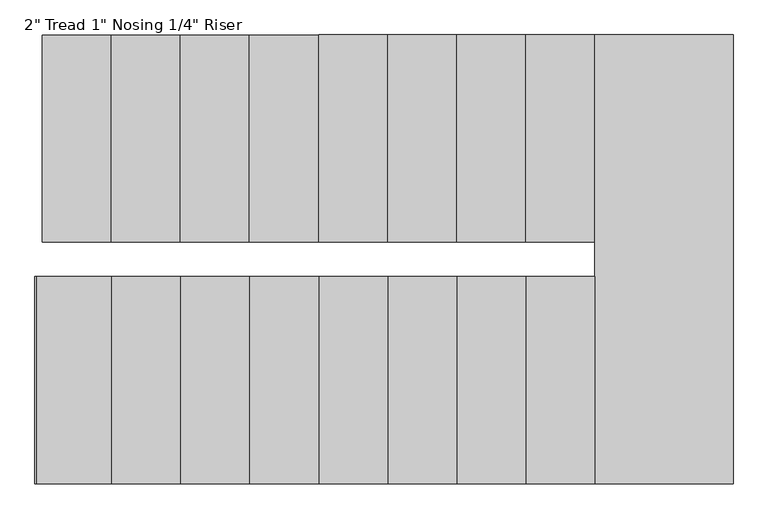
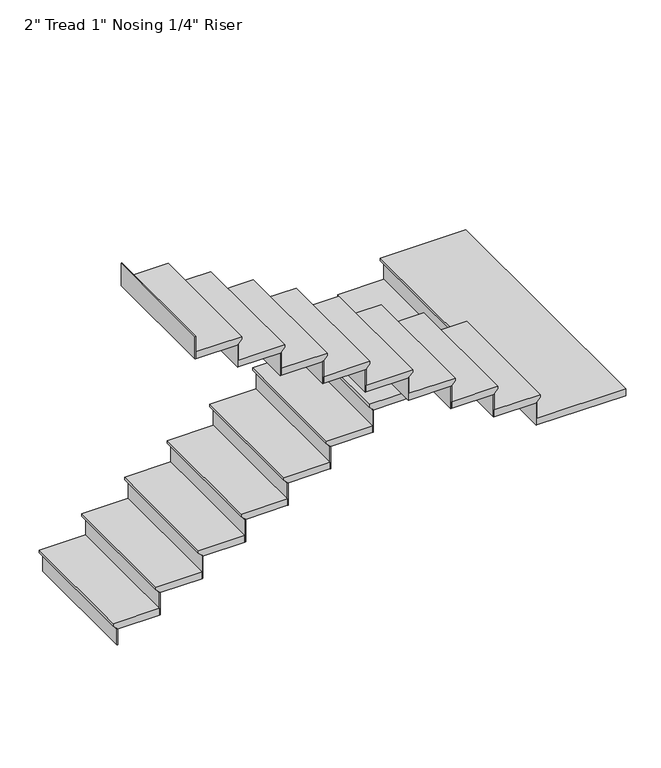
"""IFC4 building model written with IfcOpenShell, lengths in millimetres: stair flight geometry."""

from ifc_helpers import new_model, si_unit, origin, place, context, project, spatial, faceted_brep, source, transform, mapped, element, save


def stair_flight_0ccda8d3(model_context):
    return source(origin(), model_context, "Body", "Brep", [
        faceted_brep([(4699.0, 4356.1, 150.2833333), (4699.0, 4356.1, 169.3333333), (4699.0, 5270.5, 169.3333333), (4699.0, 5270.5, 150.2833333), (4724.4, 4356.1, 124.8833333), (4724.4, 5270.5, 124.8833333), (5029.2, 4356.1, 169.3333333), (5029.2, 5270.5, 169.3333333), (4724.4, 5270.5, 118.5333333), (5029.2, 5270.5, 118.5333333), (5029.2, 4356.1, 118.5333333), (4724.4, 4356.1, 118.5333333)], [[[0, 1, 2, 3]], [[4, 0, 3, 5]], [[2, 1, 6, 7]], [[8, 9, 10, 11]], [[2, 7, 9, 8, 5, 3]], [[8, 11, 4, 5]], [[6, 1, 0, 4, 11, 10]], [[7, 6, 10, 9]]]),
        faceted_brep([(4724.4, 4356.1, 118.5333333), (4724.4, 4356.1, 0.0), (4730.75, 4356.1, 0.0), (4730.75, 4356.1, 118.5333333), (4724.4, 5270.5, 118.5333333), (4730.75, 5270.5, 118.5333333), (4730.75, 5270.5, 0.0), (4724.4, 5270.5, 0.0)], [[[0, 1, 2, 3]], [[4, 5, 6, 7]], [[1, 0, 4, 7]], [[2, 1, 7, 6]], [[3, 2, 6, 5]], [[0, 3, 5, 4]]]),
        faceted_brep([(5029.2, 4356.1, 287.8666667), (5029.2, 4356.1, 118.5333333), (5035.55, 4356.1, 118.5333333), (5035.55, 4356.1, 287.8666667), (5029.2, 5270.5, 287.8666667), (5035.55, 5270.5, 287.8666667), (5035.55, 5270.5, 118.5333333), (5029.2, 5270.5, 118.5333333)], [[[0, 1, 2, 3]], [[4, 5, 6, 7]], [[1, 0, 4, 7]], [[2, 1, 7, 6]], [[3, 2, 6, 5]], [[0, 3, 5, 4]]]),
        faceted_brep([(5003.8, 5270.5, 338.6666667), (5003.8, 4356.1, 338.6666667), (5334.0, 4356.1, 338.6666667), (5334.0, 5270.5, 338.6666667), (5029.2, 5270.5, 287.8666667), (5334.0, 5270.5, 287.8666667), (5334.0, 4356.1, 287.8666667), (5029.2, 4356.1, 287.8666667), (5029.2, 5270.5, 294.2166667), (5003.8, 5270.5, 319.6166667), (5029.2, 4356.1, 294.2166667), (5003.8, 4356.1, 319.6166667)], [[[0, 1, 2, 3]], [[4, 5, 6, 7]], [[0, 3, 5, 4, 8, 9]], [[4, 7, 10, 8]], [[2, 1, 11, 10, 7, 6]], [[3, 2, 6, 5]], [[11, 1, 0, 9]], [[10, 11, 9, 8]]]),
        faceted_brep([(5334.0, 4356.1, 457.2), (5334.0, 4356.1, 287.8666667), (5340.35, 4356.1, 287.8666667), (5340.35, 4356.1, 457.2), (5334.0, 5270.5, 457.2), (5340.35, 5270.5, 457.2), (5340.35, 5270.5, 287.8666667), (5334.0, 5270.5, 287.8666667)], [[[0, 1, 2, 3]], [[4, 5, 6, 7]], [[1, 0, 4, 7]], [[2, 1, 7, 6]], [[3, 2, 6, 5]], [[0, 3, 5, 4]]]),
        faceted_brep([(5308.6, 5270.5, 508.0), (5308.6, 4356.1, 508.0), (5638.8, 4356.1, 508.0), (5638.8, 5270.5, 508.0), (5334.0, 5270.5, 457.2), (5638.8, 5270.5, 457.2), (5638.8, 4356.1, 457.2), (5334.0, 4356.1, 457.2), (5334.0, 5270.5, 463.55), (5308.6, 5270.5, 488.95), (5334.0, 4356.1, 463.55), (5308.6, 4356.1, 488.95)], [[[0, 1, 2, 3]], [[4, 5, 6, 7]], [[0, 3, 5, 4, 8, 9]], [[4, 7, 10, 8]], [[2, 1, 11, 10, 7, 6]], [[3, 2, 6, 5]], [[11, 1, 0, 9]], [[10, 11, 9, 8]]]),
        faceted_brep([(5638.8, 4356.1, 626.5333333), (5638.8, 4356.1, 457.2), (5645.15, 4356.1, 457.2), (5645.15, 4356.1, 626.5333333), (5638.8, 5270.5, 626.5333333), (5645.15, 5270.5, 626.5333333), (5645.15, 5270.5, 457.2), (5638.8, 5270.5, 457.2)], [[[0, 1, 2, 3]], [[4, 5, 6, 7]], [[1, 0, 4, 7]], [[2, 1, 7, 6]], [[3, 2, 6, 5]], [[0, 3, 5, 4]]]),
        faceted_brep([(5613.4, 5270.5, 677.3333333), (5613.4, 4356.1, 677.3333333), (5943.6, 4356.1, 677.3333333), (5943.6, 5270.5, 677.3333333), (5638.8, 5270.5, 626.5333333), (5943.6, 5270.5, 626.5333333), (5943.6, 4356.1, 626.5333333), (5638.8, 4356.1, 626.5333333), (5638.8, 5270.5, 632.8833333), (5613.4, 5270.5, 658.2833333), (5638.8, 4356.1, 632.8833333), (5613.4, 4356.1, 658.2833333)], [[[0, 1, 2, 3]], [[4, 5, 6, 7]], [[0, 3, 5, 4, 8, 9]], [[4, 7, 10, 8]], [[2, 1, 11, 10, 7, 6]], [[3, 2, 6, 5]], [[11, 1, 0, 9]], [[10, 11, 9, 8]]]),
        faceted_brep([(5943.6, 4356.1, 795.8666667), (5943.6, 4356.1, 626.5333333), (5949.95, 4356.1, 626.5333333), (5949.95, 4356.1, 795.8666667), (5943.6, 5270.5, 795.8666667), (5949.95, 5270.5, 795.8666667), (5949.95, 5270.5, 626.5333333), (5943.6, 5270.5, 626.5333333)], [[[0, 1, 2, 3]], [[4, 5, 6, 7]], [[1, 0, 4, 7]], [[2, 1, 7, 6]], [[3, 2, 6, 5]], [[0, 3, 5, 4]]]),
        faceted_brep([(5918.2, 5270.5, 846.6666667), (5918.2, 4356.1, 846.6666667), (6248.4, 4356.1, 846.6666667), (6248.4, 5270.5, 846.6666667), (5943.6, 5270.5, 795.8666667), (6248.4, 5270.5, 795.8666667), (6248.4, 4356.1, 795.8666667), (5943.6, 4356.1, 795.8666667), (5943.6, 5270.5, 802.2166667), (5918.2, 5270.5, 827.6166667), (5943.6, 4356.1, 802.2166667), (5918.2, 4356.1, 827.6166667)], [[[0, 1, 2, 3]], [[4, 5, 6, 7]], [[0, 3, 5, 4, 8, 9]], [[4, 7, 10, 8]], [[2, 1, 11, 10, 7, 6]], [[3, 2, 6, 5]], [[11, 1, 0, 9]], [[10, 11, 9, 8]]]),
        faceted_brep([(6248.4, 4356.1, 965.2), (6248.4, 4356.1, 795.8666667), (6254.75, 4356.1, 795.8666667), (6254.75, 4356.1, 965.2), (6248.4, 5270.5, 965.2), (6254.75, 5270.5, 965.2), (6254.75, 5270.5, 795.8666667), (6248.4, 5270.5, 795.8666667)], [[[0, 1, 2, 3]], [[4, 5, 6, 7]], [[1, 0, 4, 7]], [[2, 1, 7, 6]], [[3, 2, 6, 5]], [[0, 3, 5, 4]]]),
        faceted_brep([(6223.0, 5270.5, 1016.0), (6223.0, 4356.1, 1016.0), (6553.2, 4356.1, 1016.0), (6553.2, 5270.5, 1016.0), (6248.4, 5270.5, 965.2), (6553.2, 5270.5, 965.2), (6553.2, 4356.1, 965.2), (6248.4, 4356.1, 965.2), (6248.4, 5270.5, 971.55), (6223.0, 5270.5, 996.95), (6248.4, 4356.1, 971.55), (6223.0, 4356.1, 996.95)], [[[0, 1, 2, 3]], [[4, 5, 6, 7]], [[0, 3, 5, 4, 8, 9]], [[4, 7, 10, 8]], [[2, 1, 11, 10, 7, 6]], [[3, 2, 6, 5]], [[11, 1, 0, 9]], [[10, 11, 9, 8]]]),
        faceted_brep([(6553.2, 4356.1, 1134.5333333), (6553.2, 4356.1, 965.2), (6559.55, 4356.1, 965.2), (6559.55, 4356.1, 1134.5333333), (6553.2, 5270.5, 1134.5333333), (6559.55, 5270.5, 1134.5333333), (6559.55, 5270.5, 965.2), (6553.2, 5270.5, 965.2)], [[[0, 1, 2, 3]], [[4, 5, 6, 7]], [[1, 0, 4, 7]], [[2, 1, 7, 6]], [[3, 2, 6, 5]], [[0, 3, 5, 4]]]),
        faceted_brep([(6527.8, 5270.5, 1185.3333333), (6527.8, 4356.1, 1185.3333333), (6858.0, 4356.1, 1185.3333333), (6858.0, 5270.5, 1185.3333333), (6553.2, 5270.5, 1134.5333333), (6858.0, 5270.5, 1134.5333333), (6858.0, 4356.1, 1134.5333333), (6553.2, 4356.1, 1134.5333333), (6553.2, 5270.5, 1140.8833333), (6527.8, 5270.5, 1166.2833333), (6553.2, 4356.1, 1140.8833333), (6527.8, 4356.1, 1166.2833333)], [[[0, 1, 2, 3]], [[4, 5, 6, 7]], [[0, 3, 5, 4, 8, 9]], [[4, 7, 10, 8]], [[2, 1, 11, 10, 7, 6]], [[3, 2, 6, 5]], [[11, 1, 0, 9]], [[10, 11, 9, 8]]]),
        faceted_brep([(6858.0, 4356.1, 1303.8666667), (6858.0, 4356.1, 1134.5333333), (6864.35, 4356.1, 1134.5333333), (6864.35, 4356.1, 1303.8666667), (6858.0, 5270.5, 1303.8666667), (6864.35, 5270.5, 1303.8666667), (6864.35, 5270.5, 1134.5333333), (6858.0, 5270.5, 1134.5333333)], [[[0, 1, 2, 3]], [[4, 5, 6, 7]], [[1, 0, 4, 7]], [[2, 1, 7, 6]], [[3, 2, 6, 5]], [[0, 3, 5, 4]]]),
        faceted_brep([(6832.6, 5270.5, 1354.6666667), (6832.6, 4356.1, 1354.6666667), (7162.8, 4356.1, 1354.6666667), (7162.8, 5270.5, 1354.6666667), (6858.0, 5270.5, 1303.8666667), (7162.8, 5270.5, 1303.8666667), (7162.8, 4356.1, 1303.8666667), (6858.0, 4356.1, 1303.8666667), (6858.0, 5270.5, 1310.2166667), (6832.6, 5270.5, 1335.6166667), (6858.0, 4356.1, 1310.2166667), (6832.6, 4356.1, 1335.6166667)], [[[0, 1, 2, 3]], [[4, 5, 6, 7]], [[0, 3, 5, 4, 8, 9]], [[4, 7, 10, 8]], [[2, 1, 11, 10, 7, 6]], [[3, 2, 6, 5]], [[11, 1, 0, 9]], [[10, 11, 9, 8]]]),
        faceted_brep([(7162.8, 4356.1, 1473.2), (7162.8, 4356.1, 1303.8666667), (7169.15, 4356.1, 1303.8666667), (7169.15, 4356.1, 1473.2), (7162.8, 5270.5, 1473.2), (7169.15, 5270.5, 1473.2), (7169.15, 5270.5, 1303.8666667), (7162.8, 5270.5, 1303.8666667)], [[[0, 1, 2, 3]], [[4, 5, 6, 7]], [[1, 0, 4, 7]], [[2, 1, 7, 6]], [[3, 2, 6, 5]], [[0, 3, 5, 4]]]),
        faceted_brep([(7112.0, 3289.3, 1524.0), (7747.0, 3289.3, 1524.0), (7747.0, 5270.5, 1524.0), (7137.4, 5270.5, 1524.0), (7137.4, 4203.7, 1524.0), (7112.0, 4203.7, 1524.0), (7747.0, 3289.3, 1473.2), (7112.0, 3289.3, 1473.2), (7112.0, 4203.7, 1473.2), (7137.4, 4203.7, 1473.2), (7137.4, 4356.1, 1473.2), (7162.8, 4356.1, 1473.2), (7162.8, 5270.5, 1473.2), (7747.0, 5270.5, 1473.2), (7162.8, 5270.5, 1479.55), (7137.4, 5270.5, 1504.95), (7162.8, 4356.1, 1479.55), (7137.4, 4356.1, 1504.95)], [[[0, 1, 2, 3, 4, 5]], [[6, 7, 8, 9, 10, 11, 12, 13]], [[1, 0, 7, 6]], [[2, 1, 6, 13]], [[3, 2, 13, 12, 14, 15]], [[12, 11, 16, 14]], [[11, 10, 17, 16]], [[4, 3, 15, 17, 10, 9]], [[5, 4, 9, 8]], [[0, 5, 8, 7]], [[15, 14, 16, 17]]]),
        faceted_brep([(7112.0, 4203.7, 1642.5333333), (7112.0, 4203.7, 1473.2), (7105.65, 4203.7, 1473.2), (7105.65, 4203.7, 1642.5333333), (7112.0, 3289.3, 1642.5333333), (7105.65, 3289.3, 1642.5333333), (7105.65, 3289.3, 1473.2), (7112.0, 3289.3, 1473.2)], [[[0, 1, 2, 3]], [[4, 5, 6, 7]], [[1, 0, 4, 7]], [[2, 1, 7, 6]], [[3, 2, 6, 5]], [[0, 3, 5, 4]]]),
        faceted_brep([(7137.4, 3289.3, 1693.3333333), (7137.4, 4203.7, 1693.3333333), (6807.2, 4203.7, 1693.3333333), (6807.2, 3289.3, 1693.3333333), (7112.0, 3289.3, 1642.5333333), (6807.2, 3289.3, 1642.5333333), (6807.2, 4203.7, 1642.5333333), (7112.0, 4203.7, 1642.5333333), (7112.0, 3289.3, 1648.8833333), (7137.4, 3289.3, 1674.2833333), (7112.0, 4203.7, 1648.8833333), (7137.4, 4203.7, 1674.2833333)], [[[0, 1, 2, 3]], [[4, 5, 6, 7]], [[0, 3, 5, 4, 8, 9]], [[4, 7, 10, 8]], [[2, 1, 11, 10, 7, 6]], [[3, 2, 6, 5]], [[11, 1, 0, 9]], [[10, 11, 9, 8]]]),
        faceted_brep([(6807.2, 4203.7, 1811.8666667), (6807.2, 4203.7, 1642.5333333), (6800.85, 4203.7, 1642.5333333), (6800.85, 4203.7, 1811.8666667), (6807.2, 3289.3, 1811.8666667), (6800.85, 3289.3, 1811.8666667), (6800.85, 3289.3, 1642.5333333), (6807.2, 3289.3, 1642.5333333)], [[[0, 1, 2, 3]], [[4, 5, 6, 7]], [[1, 0, 4, 7]], [[2, 1, 7, 6]], [[3, 2, 6, 5]], [[0, 3, 5, 4]]]),
        faceted_brep([(6832.6, 3289.3, 1862.6666667), (6832.6, 4203.7, 1862.6666667), (6502.4, 4203.7, 1862.6666667), (6502.4, 3289.3, 1862.6666667), (6807.2, 3289.3, 1811.8666667), (6502.4, 3289.3, 1811.8666667), (6502.4, 4203.7, 1811.8666667), (6807.2, 4203.7, 1811.8666667), (6807.2, 3289.3, 1818.2166667), (6832.6, 3289.3, 1843.6166667), (6807.2, 4203.7, 1818.2166667), (6832.6, 4203.7, 1843.6166667)], [[[0, 1, 2, 3]], [[4, 5, 6, 7]], [[0, 3, 5, 4, 8, 9]], [[4, 7, 10, 8]], [[2, 1, 11, 10, 7, 6]], [[3, 2, 6, 5]], [[11, 1, 0, 9]], [[10, 11, 9, 8]]]),
        faceted_brep([(6502.4, 4203.7, 1981.2), (6502.4, 4203.7, 1811.8666667), (6496.05, 4203.7, 1811.8666667), (6496.05, 4203.7, 1981.2), (6502.4, 3289.3, 1981.2), (6496.05, 3289.3, 1981.2), (6496.05, 3289.3, 1811.8666667), (6502.4, 3289.3, 1811.8666667)], [[[0, 1, 2, 3]], [[4, 5, 6, 7]], [[1, 0, 4, 7]], [[2, 1, 7, 6]], [[3, 2, 6, 5]], [[0, 3, 5, 4]]]),
        faceted_brep([(6527.8, 3289.3, 2032.0), (6527.8, 4203.7, 2032.0), (6197.6, 4203.7, 2032.0), (6197.6, 3289.3, 2032.0), (6502.4, 3289.3, 1981.2), (6197.6, 3289.3, 1981.2), (6197.6, 4203.7, 1981.2), (6502.4, 4203.7, 1981.2), (6502.4, 3289.3, 1987.55), (6527.8, 3289.3, 2012.95), (6502.4, 4203.7, 1987.55), (6527.8, 4203.7, 2012.95)], [[[0, 1, 2, 3]], [[4, 5, 6, 7]], [[0, 3, 5, 4, 8, 9]], [[4, 7, 10, 8]], [[2, 1, 11, 10, 7, 6]], [[3, 2, 6, 5]], [[11, 1, 0, 9]], [[10, 11, 9, 8]]]),
        faceted_brep([(6197.6, 4203.7, 2150.5333333), (6197.6, 4203.7, 1981.2), (6191.25, 4203.7, 1981.2), (6191.25, 4203.7, 2150.5333333), (6197.6, 3289.3, 2150.5333333), (6191.25, 3289.3, 2150.5333333), (6191.25, 3289.3, 1981.2), (6197.6, 3289.3, 1981.2)], [[[0, 1, 2, 3]], [[4, 5, 6, 7]], [[1, 0, 4, 7]], [[2, 1, 7, 6]], [[3, 2, 6, 5]], [[0, 3, 5, 4]]]),
        faceted_brep([(6223.0, 3289.3, 2201.3333333), (6223.0, 4203.7, 2201.3333333), (5892.8, 4203.7, 2201.3333333), (5892.8, 3289.3, 2201.3333333), (6197.6, 3289.3, 2150.5333333), (5892.8, 3289.3, 2150.5333333), (5892.8, 4203.7, 2150.5333333), (6197.6, 4203.7, 2150.5333333), (6197.6, 3289.3, 2156.8833333), (6223.0, 3289.3, 2182.2833333), (6197.6, 4203.7, 2156.8833333), (6223.0, 4203.7, 2182.2833333)], [[[0, 1, 2, 3]], [[4, 5, 6, 7]], [[0, 3, 5, 4, 8, 9]], [[4, 7, 10, 8]], [[2, 1, 11, 10, 7, 6]], [[3, 2, 6, 5]], [[11, 1, 0, 9]], [[10, 11, 9, 8]]]),
        faceted_brep([(5892.8, 4203.7, 2319.8666667), (5892.8, 4203.7, 2150.5333333), (5886.45, 4203.7, 2150.5333333), (5886.45, 4203.7, 2319.8666667), (5892.8, 3289.3, 2319.8666667), (5886.45, 3289.3, 2319.8666667), (5886.45, 3289.3, 2150.5333333), (5892.8, 3289.3, 2150.5333333)], [[[0, 1, 2, 3]], [[4, 5, 6, 7]], [[1, 0, 4, 7]], [[2, 1, 7, 6]], [[3, 2, 6, 5]], [[0, 3, 5, 4]]]),
        faceted_brep([(5918.2, 3289.3, 2370.6666667), (5918.2, 4203.7, 2370.6666667), (5588.0, 4203.7, 2370.6666667), (5588.0, 3289.3, 2370.6666667), (5892.8, 3289.3, 2319.8666667), (5588.0, 3289.3, 2319.8666667), (5588.0, 4203.7, 2319.8666667), (5892.8, 4203.7, 2319.8666667), (5892.8, 3289.3, 2326.2166667), (5918.2, 3289.3, 2351.6166667), (5892.8, 4203.7, 2326.2166667), (5918.2, 4203.7, 2351.6166667)], [[[0, 1, 2, 3]], [[4, 5, 6, 7]], [[0, 3, 5, 4, 8, 9]], [[4, 7, 10, 8]], [[2, 1, 11, 10, 7, 6]], [[3, 2, 6, 5]], [[11, 1, 0, 9]], [[10, 11, 9, 8]]]),
        faceted_brep([(5588.0, 4203.7, 2489.2), (5588.0, 4203.7, 2319.8666667), (5581.65, 4203.7, 2319.8666667), (5581.65, 4203.7, 2489.2), (5588.0, 3289.3, 2489.2), (5581.65, 3289.3, 2489.2), (5581.65, 3289.3, 2319.8666667), (5588.0, 3289.3, 2319.8666667)], [[[0, 1, 2, 3]], [[4, 5, 6, 7]], [[1, 0, 4, 7]], [[2, 1, 7, 6]], [[3, 2, 6, 5]], [[0, 3, 5, 4]]]),
        faceted_brep([(5613.4, 3289.3, 2540.0), (5613.4, 4203.7, 2540.0), (5283.2, 4203.7, 2540.0), (5283.2, 3289.3, 2540.0), (5588.0, 3289.3, 2489.2), (5283.2, 3289.3, 2489.2), (5283.2, 4203.7, 2489.2), (5588.0, 4203.7, 2489.2), (5588.0, 3289.3, 2495.55), (5613.4, 3289.3, 2520.95), (5588.0, 4203.7, 2495.55), (5613.4, 4203.7, 2520.95)], [[[0, 1, 2, 3]], [[4, 5, 6, 7]], [[0, 3, 5, 4, 8, 9]], [[4, 7, 10, 8]], [[2, 1, 11, 10, 7, 6]], [[3, 2, 6, 5]], [[11, 1, 0, 9]], [[10, 11, 9, 8]]]),
        faceted_brep([(5283.2, 4203.7, 2658.5333333), (5283.2, 4203.7, 2489.2), (5276.85, 4203.7, 2489.2), (5276.85, 4203.7, 2658.5333333), (5283.2, 3289.3, 2658.5333333), (5276.85, 3289.3, 2658.5333333), (5276.85, 3289.3, 2489.2), (5283.2, 3289.3, 2489.2)], [[[0, 1, 2, 3]], [[4, 5, 6, 7]], [[1, 0, 4, 7]], [[2, 1, 7, 6]], [[3, 2, 6, 5]], [[0, 3, 5, 4]]]),
        faceted_brep([(5308.6, 3289.3, 2709.3333333), (5308.6, 4203.7, 2709.3333333), (4978.4, 4203.7, 2709.3333333), (4978.4, 3289.3, 2709.3333333), (5283.2, 3289.3, 2658.5333333), (4978.4, 3289.3, 2658.5333333), (4978.4, 4203.7, 2658.5333333), (5283.2, 4203.7, 2658.5333333), (5283.2, 3289.3, 2664.8833333), (5308.6, 3289.3, 2690.2833333), (5283.2, 4203.7, 2664.8833333), (5308.6, 4203.7, 2690.2833333)], [[[0, 1, 2, 3]], [[4, 5, 6, 7]], [[0, 3, 5, 4, 8, 9]], [[4, 7, 10, 8]], [[2, 1, 11, 10, 7, 6]], [[3, 2, 6, 5]], [[11, 1, 0, 9]], [[10, 11, 9, 8]]]),
        faceted_brep([(4978.4, 4203.7, 2827.8666667), (4978.4, 4203.7, 2658.5333333), (4972.05, 4203.7, 2658.5333333), (4972.05, 4203.7, 2827.8666667), (4978.4, 3289.3, 2827.8666667), (4972.05, 3289.3, 2827.8666667), (4972.05, 3289.3, 2658.5333333), (4978.4, 3289.3, 2658.5333333)], [[[0, 1, 2, 3]], [[4, 5, 6, 7]], [[1, 0, 4, 7]], [[2, 1, 7, 6]], [[3, 2, 6, 5]], [[0, 3, 5, 4]]]),
        faceted_brep([(4673.6, 4203.7, 2997.2), (4673.6, 4203.7, 2827.8666667), (4667.25, 4203.7, 2827.8666667), (4667.25, 4203.7, 2997.2), (4673.6, 3289.3, 2997.2), (4667.25, 3289.3, 2997.2), (4667.25, 3289.3, 2827.8666667), (4673.6, 3289.3, 2827.8666667)], [[[0, 1, 2, 3]], [[4, 5, 6, 7]], [[1, 0, 4, 7]], [[2, 1, 7, 6]], [[3, 2, 6, 5]], [[0, 3, 5, 4]]]),
        faceted_brep([(5003.8, 3289.3, 2878.6666667), (5003.8, 4203.7, 2878.6666667), (4673.6, 4203.7, 2878.6666667), (4673.6, 3289.3, 2878.6666667), (4978.4, 3289.3, 2827.8666667), (4673.6, 3289.3, 2827.8666667), (4673.6, 4203.7, 2827.8666667), (4978.4, 4203.7, 2827.8666667), (4978.4, 3289.3, 2834.2166667), (5003.8, 3289.3, 2859.6166667), (4978.4, 4203.7, 2834.2166667), (5003.8, 4203.7, 2859.6166667)], [[[0, 1, 2, 3]], [[4, 5, 6, 7]], [[0, 3, 5, 4, 8, 9]], [[4, 7, 10, 8]], [[2, 1, 11, 10, 7, 6]], [[3, 2, 6, 5]], [[11, 1, 0, 9]], [[10, 11, 9, 8]]]),
    ])


if __name__ == "__main__":
    model = new_model("IFC4")
    model_context = context("Model", 3, world=origin())
    ifc_project = project(units=[si_unit("LENGTHUNIT", "METRE", prefix="MILLI")], contexts=[model_context])
    site = spatial("IfcSite", under=ifc_project)
    building = spatial("IfcBuilding", under=site)
    placement = place(None, origin())
    stair_flight_shape = stair_flight_0ccda8d3(model_context)
    element("IfcStairFlight", 1, ObjectType="2\" Tread 1\" Nosing 1/4\" Riser", at=placement, inside=building, context=model_context, shape_type="MappedRepresentation", body=[
        mapped(stair_flight_shape, transform((0.0, 0.0, 0.0), x_axis=(1.0, 0.0, 0.0), y_axis=(0.0, 1.0, 0.0), z_axis=(0.0, 0.0, 1.0))),
    ])
    save(model, "model.ifc")
